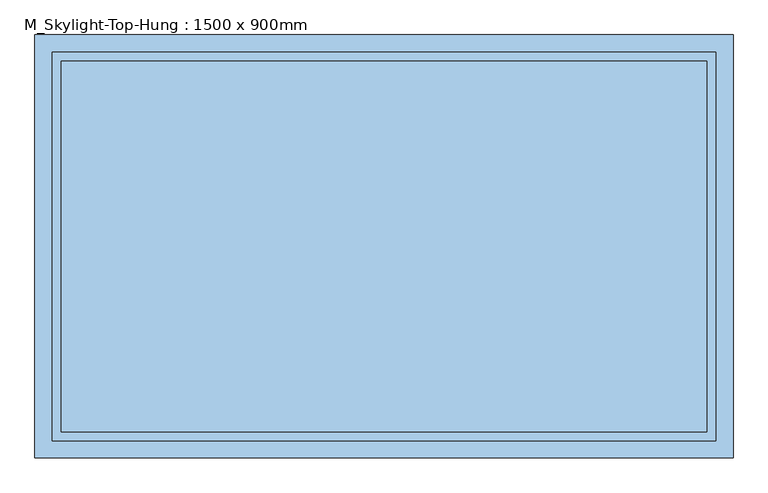
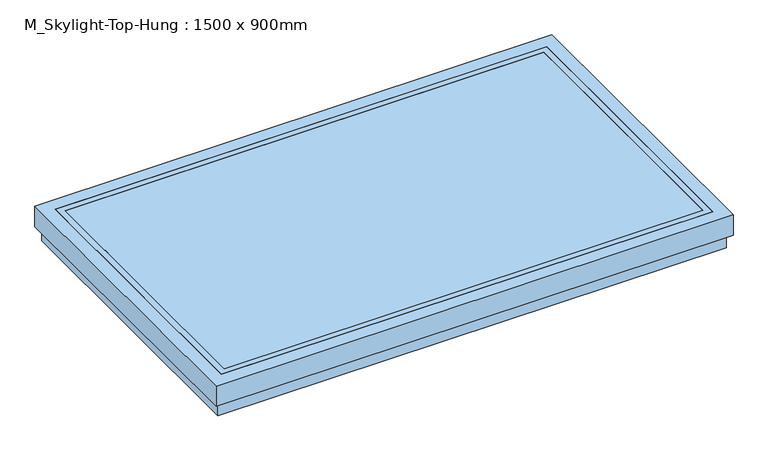
"""IFC4 building model written with IfcOpenShell, lengths in millimetres: window geometry, M_Skylight-Top-Hung : 1500 x 900mm."""

from ifc_helpers import new_model, si_unit, frame, origin, place, context, project, spatial, polyline, outline, extrude, faceted_brep, source, transform, mapped, element, save


def m_skylight_top_hung_1500_x_900mm_68f14329(model_context):
    return source(origin(), model_context, "Body", "SolidModel", [
        faceted_brep([(750.0, 450.0, 3962.4), (750.0, 450.0, 4042.4), (750.0, -450.0, 4042.4), (750.0, -450.0, 3962.4), (686.5, 386.5, 4017.0), (686.5, 386.5, 3962.4), (686.5, -386.5, 3962.4), (686.5, -386.5, 4017.0), (724.6, 424.6, 4042.4), (724.6, 424.6, 4017.0), (724.6, -424.6, 4017.0), (724.6, -424.6, 4042.4), (-750.0, -450.0, 4042.4), (-750.0, -450.0, 3962.4), (-686.5, -386.5, 3962.4), (-686.5, -386.5, 4017.0), (-724.6, -424.6, 4017.0), (-724.6, -424.6, 4042.4), (-750.0, 450.0, 4042.4), (-750.0, 450.0, 3962.4), (-686.5, 386.5, 3962.4), (-686.5, 386.5, 4017.0), (-724.6, 424.6, 4017.0), (-724.6, 424.6, 4042.4)], [[[0, 1, 2, 3]], [[4, 5, 6, 7]], [[8, 9, 10, 11]], [[3, 2, 12, 13]], [[7, 6, 14, 15]], [[11, 10, 16, 17]], [[13, 12, 18, 19]], [[15, 14, 20, 21]], [[17, 16, 22, 23]], [[19, 18, 1, 0]], [[3, 13, 19, 0], [5, 20, 14, 6]], [[21, 20, 5, 4]], [[9, 22, 16, 10], [7, 15, 21, 4]], [[23, 22, 9, 8]], [[1, 18, 12, 2], [11, 17, 23, 8]]]),
        faceted_brep([(762.7, 462.7, 4004.3), (762.7, 462.7, 4067.8), (762.7, -462.7, 4067.8), (762.7, -462.7, 4004.3), (750.0, 450.0, 4042.4), (750.0, 450.0, 4004.3), (750.0, -450.0, 4004.3), (750.0, -450.0, 4042.4), (724.6, 424.6, 4067.8), (724.6, 424.6, 4042.4), (724.6, -424.6, 4042.4), (724.6, -424.6, 4067.8), (-762.7, -462.7, 4067.8), (-762.7, -462.7, 4004.3), (-750.0, -450.0, 4004.3), (-750.0, -450.0, 4042.4), (-724.6, -424.6, 4042.4), (-724.6, -424.6, 4067.8), (-762.7, 462.7, 4067.8), (-762.7, 462.7, 4004.3), (-750.0, 450.0, 4004.3), (-750.0, 450.0, 4042.4), (-724.6, 424.6, 4042.4), (-724.6, 424.6, 4067.8)], [[[0, 1, 2, 3]], [[4, 5, 6, 7]], [[8, 9, 10, 11]], [[3, 2, 12, 13]], [[7, 6, 14, 15]], [[11, 10, 16, 17]], [[13, 12, 18, 19]], [[15, 14, 20, 21]], [[17, 16, 22, 23]], [[1, 18, 12, 2], [11, 17, 23, 8]], [[19, 18, 1, 0]], [[3, 13, 19, 0], [5, 20, 14, 6]], [[21, 20, 5, 4]], [[7, 15, 21, 4], [9, 22, 16, 10]], [[23, 22, 9, 8]]]),
        extrude(outline(polyline([(705.55, 405.55), (705.55, -405.55), (-705.55, -405.55), (-705.55, 405.55), (705.55, 405.55)])), frame((0.0, 0.0, 4062.24375), z_axis=(0.0, 0.0, 1.0), x_axis=(1.0, 0.0, 0.0)), (0.0, 0.0, 1.0), 5.55625),
        faceted_brep([(724.6, 424.6, 4017.0), (724.6, 424.6, 4067.8), (724.6, -424.6, 4067.8), (724.6, -424.6, 4017.0), (686.5, 386.5, 4048.75), (686.5, 386.5, 4017.0), (686.5, -386.5, 4017.0), (686.5, -386.5, 4048.75), (705.55, 405.55, 4067.8), (705.55, 405.55, 4048.75), (705.55, -405.55, 4048.75), (705.55, -405.55, 4067.8), (-724.6, -424.6, 4067.8), (-724.6, -424.6, 4017.0), (-686.5, -386.5, 4017.0), (-686.5, -386.5, 4048.75), (-705.55, -405.55, 4048.75), (-705.55, -405.55, 4067.8), (-724.6, 424.6, 4067.8), (-724.6, 424.6, 4017.0), (-686.5, 386.5, 4017.0), (-686.5, 386.5, 4048.75), (-705.55, 405.55, 4048.75), (-705.55, 405.55, 4067.8)], [[[0, 1, 2, 3]], [[4, 5, 6, 7]], [[8, 9, 10, 11]], [[3, 2, 12, 13]], [[7, 6, 14, 15]], [[11, 10, 16, 17]], [[13, 12, 18, 19]], [[15, 14, 20, 21]], [[17, 16, 22, 23]], [[1, 18, 12, 2], [11, 17, 23, 8]], [[19, 18, 1, 0]], [[3, 13, 19, 0], [5, 20, 14, 6]], [[21, 20, 5, 4]], [[9, 22, 16, 10], [7, 15, 21, 4]], [[23, 22, 9, 8]]]),
    ])


if __name__ == "__main__":
    model = new_model("IFC4")
    model_context = context("Model", 3, world=origin())
    ifc_project = project(units=[si_unit("LENGTHUNIT", "METRE", prefix="MILLI")], contexts=[model_context])
    site = spatial("IfcSite", under=ifc_project)
    building = spatial("IfcBuilding", under=site)
    placement = place(None, origin())
    m_skylight_top_hung_1500_x_900mm_shape = m_skylight_top_hung_1500_x_900mm_68f14329(model_context)
    element("IfcWindow", 1, ObjectType="M_Skylight-Top-Hung : 1500 x 900mm", at=placement, inside=building, context=model_context, shape_type="MappedRepresentation", body=[
        mapped(m_skylight_top_hung_1500_x_900mm_shape, transform((0.0, 0.0, 0.0), x_axis=(1.0, 0.0, 0.0), y_axis=(0.0, 1.0, 0.0), z_axis=(0.0, 0.0, 1.0))),
    ])
    save(model, "model.ifc")

# Revit data of these elements
# Type "M_Skylight-Top-Hung : 1500 x 900mm"
#   Type Mark = "23"
#   Fire Rating = "0.5h"
#   Assembly Code = "B2020100"
#   Analytic Construction = "Single-glazed windows - domestic"
#   Width = 4' - 11.05512"
#   Visual Light Transmittance = 0.9
#   Thermal Resistance (R) = 0.9899 (h·ft²·°F)/BTU
#   Solar Heat Gain Coefficient = 0.86
#   Rough Width = 4' - 11.64567"
#   Rough Height = 3' - 0.02362"
#   Height = 2' - 11.43307"
#   Heat Transfer Coefficient (U) = 1.0102 BTU/(h·ft²·°F)
#   Base Height = 0' - 3.14961"
#   Glass Panel Material = Glass
#   Frame Material = Metal - Bronze, Light Brush
# Element 1 (IfcWindow, "M_Skylight-Top-Hung : 1500 x 900mm")
#   Materials on its faces: "Metal - Bronze, Light Brush", "Glass"
# Materials
#   "Glass": class "Glass", colour RGB 0 128 192, transparency 0.75, Description = "Soda Lime Glass", Cost = 0
#   "Metal - Bronze, Light Brush": class "Metal", colour RGB 113 80 70, transparency 0
